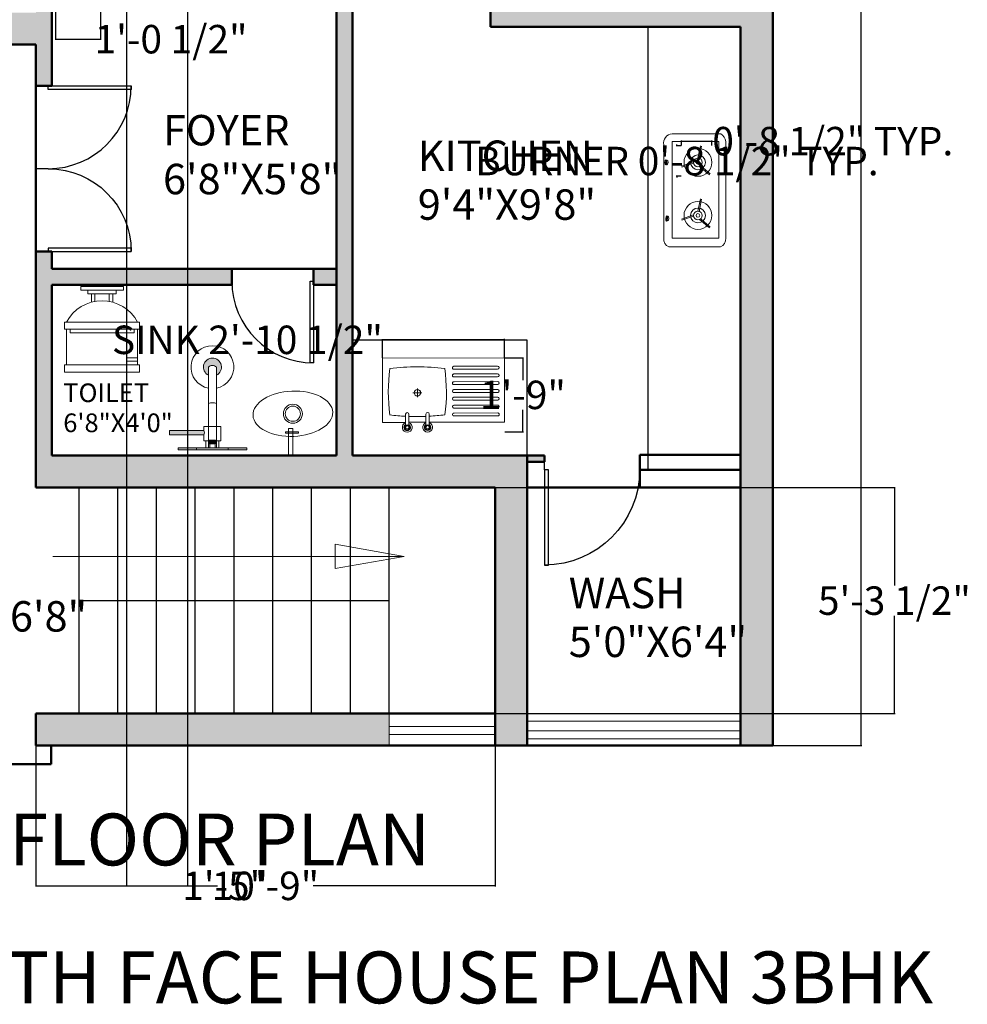
# Model space of a CAD drawing. Units: inches. Extents: x 22042254 to 25404563, y 17568978 to 17626777.
# Tile 36 of 45: x 22179932 to 22180198, y 17626125 to 17626402. Entities that reach past the tile are written whole.
import ezdxf

# ---------------------------------------------------------------- set-up
doc = ezdxf.new("R2010")
doc.units = ezdxf.units.IN
doc.header["$MEASUREMENT"] = 0
for name, color, linetype, lineweight in [('A-ANNO-DIMS', 2, 'Continuous', 18), ('A-ANNO-SYMB', 7, 'Continuous', 18), ('A-AREA-IDEN', 7, 'Continuous', 18), ('A-EQPM', 8, 'Continuous', 18), ('A-FLOR-CASE', 8, 'Continuous', 25), ('A-FLOR-STRS', 252, 'Continuous', 25), ('A-GLAZ', 4, 'Continuous', 18), ('A-WALL-PATT', 244, 'Continuous', 13), ('doors', 4, 'Continuous', 25), ('furniture', 8, 'Continuous', 18), ('PLUMBING FIXTURES', 9, 'Continuous', 18), ('text', 7, 'Continuous', 25), ('walls', 252, 'Continuous', 50)]:
    doc.layers.add(name, color=color, linetype=linetype, lineweight=lineweight)
doc.styles.get("Standard").update_dxf_attribs({"font": 'arial.ttf'})
doc.dimstyles.get("Standard").update_dxf_attribs({"dimtxt": 8, "dimasz": 0.18, "dimexe": 0.18, "dimexo": 0.0625, "dimgap": 0.09, "dimtad": 0, "dimtih": 1, "dimtoh": 1, "dimzin": 0, "dimdsep": 46, "dimlunit": 3, "dimtxsty": 'Standard', "dimcen": 0.09, "dimadec": 0, "dimazin": 0, "dimtfac": 1, "dimtofl": 0, "dimtmove": 0, "dimatfit": 3, "dimfxl": 1, "dimtolj": 1, "dimtzin": 0, "dimarcsym": 0})

# ---------------------------------------------------------------- blocks, each defined once
blk = doc.blocks.new('*D2')
at = {"layer": 'A-ANNO-DIMS', "color": 0, "lineweight": -2, "transparency": 16777216}
for p, q in [((22180143.8, 17626737.78), (22180168.82, 17626737.78)), ((22180168.64, 17626737.6), (22180168.64, 17626471.94)), ((22180168.64, 17626197.96), (22180168.64, 17626463.62)), ((22180143.8, 17626197.78), (22180168.82, 17626197.78))]:
    blk.add_line(p, q, dxfattribs=at)
at = {"layer": 'A-ANNO-DIMS', "color": 0, "transparency": 16777216}
for points in [[(22180168.61, 17626737.6), (22180168.67, 17626737.6), (22180168.64, 17626737.78)], [(22180168.61, 17626197.96), (22180168.67, 17626197.96), (22180168.64, 17626197.78)]]:
    blk.add_solid(points, dxfattribs=at)
at = {"layer": 'Defpoints', "color": 0, "transparency": 16777216}
for p in [(22180143.73, 17626737.78), (22180168.64, 17626737.78), (22180143.73, 17626197.78)]:
    blk.add_point(p, dxfattribs=at)
at = {"layer": 'A-ANNO-DIMS', "color": 0, "transparency": 16777216, "insert": (22180168.64, 17626467.78), "char_height": 8, "attachment_point": 5}
blk.add_mtext("\\A1;45'", dxfattribs=at)
blk = doc.blocks.new('A$C799204C7')
for p, q in [((0, 34.2), (17.99, 34.2)), ((0, 0), (0, 34.2)), ((17.99, 13.08), (17.99, 34.2)), ((2.32, 20.01), (2.32, 32.27)), ((3.13, 20.01), (3.13, 32.27)), ((4.48, 20.01), (4.48, 32.27)), ((5.29, 20.01), (5.29, 32.27)), ((6.64, 20.01), (6.64, 32.27)), ((7.45, 20.01), (7.45, 32.27)), ((8.85, 20.01), (8.85, 32.27)), ((9.66, 20.01), (9.66, 32.27)), ((11.01, 20.01), (11.01, 32.27)), ((11.82, 20.01), (11.82, 32.27)), ((13.22, 20.01), (13.22, 32.27)), ((14.03, 20.01), (14.03, 32.27)), ((15.42, 20.01), (15.42, 32.27)), ((16.24, 20.01), (16.24, 32.27)), ((18.59, 13.08), (15.71, 13.08)), ((15.71, 12.17), (18.59, 12.17)), ((17.99, 7.36), (17.99, 12.17)), ((8.52, 9.77), (10.9, 9.77)), ((9.73, 11), (9.73, 8.54)), ((18.59, 7.36), (15.71, 7.36)), ((15.71, 6.45), (18.59, 6.45)), ((17.99, 0), (17.99, 6.45)), ((0, 0), (17.99, 0))]:
    blk.add_line(p, q)
for centre, radius in [((19.38, 12.62), 0.684), ((19.38, 12.62), 0.456), ((9.7, 9.77), 0.916), ((19.38, 6.91), 0.684), ((19.38, 6.91), 0.456)]:
    blk.add_circle(centre, radius)
for centre, radius, start, end in [((2.72, 32.27), 0.407, 0, 180), ((4.88, 32.27), 0.407, 0, 180), ((7.05, 32.27), 0.407, 0, 180), ((9.25, 32.27), 0.407, 0, 180), ((11.42, 32.27), 0.407, 0, 180), ((13.62, 32.27), 0.407, 0, 180), ((15.83, 32.27), 0.407, 0, 180), ((2.72, 20.01), 0.407, 180, 0), ((4.88, 20.01), 0.407, 180, 0), ((7.05, 20.01), 0.407, 180, 0), ((9.25, 20.01), 0.407, 180, 0), ((11.42, 20.01), 0.407, 180, 0), ((13.62, 20.01), 0.407, 180, 0), ((15.83, 20.01), 0.407, 180, 0), ((67.33, 9.77), 64.88, 173.1952, 186.8048), ((9.53, -30.19), 48.1, 82.3437, 97.8966), ((-48.51, 9.77), 64.88, 2.9208, 6.8048), ((19.38, 12.62), 1.37, 199.6514, 160.3603), ((15.71, 12.62), 0.456, 90, 270), ((-48.51, 9.77), 64.88, 357.8723, 2.115), ((19.38, 12.62), 0.911, 210.3431, 149.7554), ((19.38, 6.91), 1.37, 199.6514, 160.3603), ((15.71, 6.91), 0.456, 90, 270), ((-48.51, 9.77), 64.88, 353.1952, 357.0665), ((19.38, 6.91), 0.911, 210.3431, 149.7554), ((9.53, 49.73), 48.1, 262.1034, 277.6563)]:
    blk.add_arc(centre, radius, start, end)
blk = doc.blocks.new('sink')
at = {"layer": 'furniture'}
for p, q in [((8718164203.894819, -1433730582.369047), (8718164201.504578, -1433730582.369047)), ((8718164202.684322, -1433730581.131674), (8718164202.684322, -1433730583.598095)), ((8718164196.150837, -1433730592.638258), (8718164196.150837, -1433730604.938997)), ((8718164196.967728, -1433730592.638258), (8718164196.967728, -1433730604.938997)), ((8718164198.365185, -1433730592.638258), (8718164198.365185, -1433730604.938997)), ((8718164199.182076, -1433730592.638258), (8718164199.182076, -1433730604.938997)), ((8718164200.579533, -1433730592.638258), (8718164200.579533, -1433730604.938997)), ((8718164201.396423, -1433730592.638258), (8718164201.396423, -1433730604.938997)), ((8718164202.748692, -1433730592.638258), (8718164202.748692, -1433730604.938997)), ((8718164203.565582, -1433730592.638258), (8718164203.565582, -1433730604.938997)), ((8718164204.963041, -1433730592.638258), (8718164204.963041, -1433730604.938997)), ((8718164205.779934, -1433730592.638258), (8718164205.779934, -1433730604.938997)), ((8718164207.1322, -1433730592.638258), (8718164207.1322, -1433730604.938997)), ((8718164207.949093, -1433730592.638258), (8718164207.949093, -1433730604.938997)), ((8718164209.301359, -1433730592.638258), (8718164209.301359, -1433730604.938997)), ((8718164210.118252, -1433730592.638258), (8718164210.118252, -1433730604.938997))]:
    blk.add_line(p, q, dxfattribs=at)
for centre, radius in [((8718164192.998869, -1433730579.495552), 0.685789), ((8718164192.998869, -1433730579.495552), 0.457192), ((8718164202.715019, -1433730582.369047), 0.919003), ((8718164192.998869, -1433730585.228166), 0.68579), ((8718164192.998869, -1433730585.228166), 0.68579), ((8718164192.998869, -1433730585.228166), 0.457192)]:
    blk.add_circle(centre, radius, dxfattribs=at)
for centre, radius, start, end in [((8718164196.559284, -1433730592.638258), 0.41045, 354.3355999, 185.6644001), ((8718164198.77363, -1433730592.638258), 0.41045, 354.3355999, 185.6644001), ((8718164200.98798, -1433730592.638258), 0.41045, 354.3355999, 185.6644001), ((8718164203.157139, -1433730592.638258), 0.41045, 354.3355999, 185.6644001), ((8718164205.371487, -1433730592.638258), 0.41045, 354.3355999, 185.6644001), ((8718164207.540646, -1433730592.640262), 0.41045, 354.3355999, 185.6644001), ((8718164209.709805, -1433730592.640262), 0.41045, 354.3355999, 185.6644001), ((8718164196.559284, -1433730604.938997), 0.408445, 180, 0), ((8718164198.77363, -1433730604.938997), 0.408445, 180, 0), ((8718164200.98798, -1433730604.938997), 0.408445, 180, 0), ((8718164203.157139, -1433730604.938997), 0.408445, 180, 0), ((8718164205.371487, -1433730604.938997), 0.408445, 180, 0), ((8718164207.540646, -1433730604.938997), 0.408445, 180, 0), ((8718164209.709805, -1433730604.938997), 0.408445, 180, 0)]:
    blk.add_arc(centre, radius, start, end, dxfattribs=at)
at = {"layer": 'furniture', "xscale": 1.0032, "yscale": 1.0032, "zscale": 1.0032, "rotation": 180}
blk.add_blockref('A$C799204C7', (8718164212.441259, -1433730572.566334), dxfattribs=at)
blk = doc.blocks.new('washbasin')
at = {"layer": 'furniture'}
blk.add_blockref('sink', (-8718164214.119328, 1433730589.721069), dxfattribs=at)
blk = doc.blocks.new('O.H SHOWER-PL')
at = {"layer": 'PLUMBING FIXTURES'}
for points in [[(-1.84, 0), (-1.84, -0.25), (1.84, -0.25), (1.84, 0)], [(0.46, -8.72), (0.46, -9.67, -0.422337), (-0.46, -9.67), (-0.46, -8.72, 4.325472)]]:
    blk.add_hatch(color=256, dxfattribs=at).paths.add_polyline_path(points)
for p, q in [((-1.84, 0), (-1.84, -0.25)), ((1.84, 0), (-1.84, 0)), ((1.84, 0), (1.84, -0.25)), ((1.84, -0.25), (-1.84, -0.25)), ((-0.46, -0.25), (-0.46, -9.67)), ((0.46, -0.25), (0.46, -9.67))]:
    blk.add_line(p, q, dxfattribs=at)
for centre, radius, start, end in [((0, -4.48), 1.03, 243.53, 296.47), ((0, -9.67), 2.5, 100.61, 79.39), ((0, -9.67), 1.05, 116.0349, 63.9652), ((0, -9.22), 0.643, 224.2078, 315.7922)]:
    blk.add_arc(centre, radius, start, end, dxfattribs=at)
blk = doc.blocks.new('DIVERTER-PL')
at = {"layer": 'PLUMBING FIXTURES'}
for points in [[(4, 0), (-4, 0), (-4, -0.25), (4, -0.25)], [(0.38, -1.14), (0.38, -0.7), (-0.37, -0.7), (-0.37, -1.14)], [(1, -1.75, 0.30818), (1, -2.25), (5, -2.25), (5, -1.75)]]:
    blk.add_hatch(color=256, dxfattribs=at).paths.add_polyline_path(points)
for p, q in [((-4, 0), (-4, -0.25)), ((-4, 0), (4, 0)), ((4, 0), (4, -0.25)), ((-4, -0.25), (4, -0.25)), ((-4, -0.25), (4, -0.25)), ((-1, -1.05), (-0.37, -1.05)), ((-1, -1.05), (-1, -2.75)), ((-0.75, -0.25), (-0.75, -1.05)), ((-0.37, -0.7), (0.38, -0.7)), ((-0.37, -0.7), (-0.37, -1.14)), ((-0.37, -1.14), (0.38, -1.14)), ((-0.32, -0.7), (-0.32, -0.25)), ((0.32, -0.7), (0.32, -0.25)), ((0.38, -0.7), (0.38, -1.14)), ((0.38, -1.05), (1, -1.05)), ((0.75, -0.25), (0.75, -1.05)), ((1, -1.05), (1, -1.75)), ((1, -2.25), (1, -2.75)), ((-1, -2.75), (1, -2.75))]:
    blk.add_line(p, q, dxfattribs=at)
at = {"layer": 'PLUMBING FIXTURES', "ltscale": 12}
for p, q in [((1, -1.75), (5, -1.75)), ((1, -2.25), (5, -2.25)), ((5, -2.25), (5, -1.75))]:
    blk.add_line(p, q, dxfattribs=at)
at = {"layer": 'PLUMBING FIXTURES'}
blk.add_arc((1.37, -2), 0.444, 145.7435, 214.2565, dxfattribs=at)
blk = doc.blocks.new('A$C7F153053')
at = {"layer": 'PLUMBING FIXTURES', "xscale": -1, "rotation": 270}
for name in ['DIVERTER-PL', 'O.H SHOWER-PL']:
    blk.add_blockref(name, (12.17, 4), dxfattribs=at)
blk = doc.blocks.new('Toilet - Imperial')
for p, q in [((-10, 22), (-10, 12)), ((-10, 21), (-7, 21)), ((-7, 20), (-10, 20)), ((-7, 21), (-7, 20)), ((10, 12), (10, 22)), ((10.5, 12), (-10.5, 12)), ((-10.5, 10), (-10.5, 12)), ((9, 13), (-9, 13)), ((-9, 13), (-9, 12)), ((9, 12), (9, 13)), ((10.5, 12), (10.5, 10)), ((10.5, 10), (-10.5, 10)), ((-3, 4.4065), (-3, 2)), ((-2, 2), (-2, 4.1658)), ((2, 4.1658), (2, 2)), ((3, 2), (3, 4.4065)), ((4, 2), (-4, 2)), ((-4, 2), (-4, 1)), ((4, 1), (4, 2))]:
    blk.add_line(p, q)
for points in [[(10.5, 22), (10.5, 24), (-10.5, 24), (-10.5, 22)], [(6, 0), (6, 1), (-6, 1), (-6, 0)]]:
    blk.add_lwpolyline(points, close=True)
blk.add_arc((0, 15.3333), 11.3333, 208.0725, 331.9275)
blk = doc.blocks.new('*U24')
for p, q in [((0, 0), (0, -6)), ((40, 0), (40, -6))]:
    blk.add_line(p, q)
blk.add_lwpolyline([(0, 0), (0, 40), (1.75, 40), (1.75, 0)], close=True)
blk.add_arc((0, 0), 40, 0, 90)
blk = doc.blocks.new('BASIN-OVAL-WITH-TAP')
for p, q in [((-11.77, 0), (-4.13, 0)), ((-5.47, 1.62), (-5.47, -2.04)), ((-5.06, 1.61), (-5.47, 1.61)), ((-5.06, -2.04), (-5.06, 1.61)), ((-4.13, 0), (-4.13, -1.24)), ((-4.13, -1.24), (-11.77, -1.24)), ((-5.47, -2.04), (-5.06, -2.04))]:
    blk.add_line(p, q)
for radius in [2.67, 2.13, 2.13, 2.13]:
    blk.add_circle((0, 0), radius)
blk.add_ellipse((0, 0), major_axis=(-0.46, -11.19), ratio=0.56899)
blk = doc.blocks.new('HOB-BURNER')
for p, q in [((0, 1.23), (0.68, 4.68)), ((0.33, 1.05), (0.97, 4.6)), ((-1.21, 0.17), (-4.61, -1.05)), ((-1.21, -0.2), (-4.53, -1.34)), ((0.46, -1.13), (3.22, -3.47)), ((0.78, -0.94), (3.43, -3.25))]:
    blk.add_line(p, q)
for radius in [3.91, 2.08, 1.22, 0.507]:
    blk.add_circle((0, 0), radius)
blk = doc.blocks.new('*D41')
at = {"layer": 'A-ANNO-DIMS', "color": 0, "lineweight": -2, "transparency": 16777216}
for p, q in [((22179942.23, 17626405.18), (22179942.23, 17626396.12)), ((22179954.87, 17626405.18), (22179954.87, 17626396.12)), ((22179942.41, 17626396.3), (22179954.69, 17626396.3)), ((22179954.87, 17626396.3), (22179955.05, 17626396.3))]:
    blk.add_line(p, q, dxfattribs=at)
at = {"layer": 'A-ANNO-DIMS', "color": 0, "transparency": 16777216}
for points in [[(22179942.41, 17626396.33), (22179942.41, 17626396.27), (22179942.23, 17626396.3)], [(22179954.69, 17626396.33), (22179954.69, 17626396.27), (22179954.87, 17626396.3)]]:
    blk.add_solid(points, dxfattribs=at)
at = {"layer": 'Defpoints', "color": 0, "transparency": 16777216}
for p in [(22179942.23, 17626405.24), (22179954.87, 17626405.24), (22179954.87, 17626396.3)]:
    blk.add_point(p, dxfattribs=at)
at = {"layer": 'A-ANNO-DIMS', "color": 0, "transparency": 16777216, "insert": (22179974.71, 17626396.3), "char_height": 8, "attachment_point": 5}
blk.add_mtext('\\A1;1\'-0 1/2"', dxfattribs=at)
blk = doc.blocks.new('*D54')
at = {"layer": 'A-ANNO-DIMS', "color": 0, "lineweight": -2, "transparency": 16777216}
for p, q in [((22180116.84, 17626366.54), (22180116.84, 17626366.72)), ((22180118.06, 17626366.36), (22180116.66, 17626366.36)), ((22180118.06, 17626357.77), (22180116.66, 17626357.77)), ((22180116.84, 17626357.59), (22180116.84, 17626357.41))]:
    blk.add_line(p, q, dxfattribs=at)
at = {"layer": 'A-ANNO-DIMS', "color": 0, "transparency": 16777216}
for points in [[(22180116.81, 17626366.54), (22180116.87, 17626366.54), (22180116.84, 17626366.36)], [(22180116.81, 17626357.59), (22180116.87, 17626357.59), (22180116.84, 17626357.77)]]:
    blk.add_solid(points, dxfattribs=at)
at = {"layer": 'Defpoints', "color": 0, "transparency": 16777216}
for p in [(22180116.84, 17626366.36), (22180118.13, 17626366.36), (22180118.13, 17626357.77)]:
    blk.add_point(p, dxfattribs=at)
at = {"layer": 'A-ANNO-DIMS', "color": 0, "transparency": 16777216, "insert": (22180116.84, 17626362.06), "char_height": 8, "attachment_point": 5}
blk.add_mtext('\\A1;BURNER 0\'-8 1/2" TYP.', dxfattribs=at)
blk = doc.blocks.new('*D55')
at = {"layer": 'A-ANNO-DIMS', "color": 0, "lineweight": -2, "transparency": 16777216}
for p, q in [((22180118.13, 17626366.42), (22180118.13, 17626367.83)), ((22180118.31, 17626367.65), (22180126.47, 17626367.65)), ((22180126.65, 17626366.42), (22180126.65, 17626367.83)), ((22180126.65, 17626367.65), (22180126.83, 17626367.65))]:
    blk.add_line(p, q, dxfattribs=at)
at = {"layer": 'A-ANNO-DIMS', "color": 0, "transparency": 16777216}
for points in [[(22180118.31, 17626367.68), (22180118.31, 17626367.62), (22180118.13, 17626367.65)], [(22180126.47, 17626367.68), (22180126.47, 17626367.62), (22180126.65, 17626367.65)]]:
    blk.add_solid(points, dxfattribs=at)
at = {"layer": 'Defpoints', "color": 0, "transparency": 16777216}
for p in [(22180126.65, 17626367.65), (22180118.13, 17626366.36), (22180126.65, 17626366.36)]:
    blk.add_point(p, dxfattribs=at)
at = {"layer": 'A-ANNO-DIMS', "color": 0, "transparency": 16777216, "insert": (22180160.62, 17626367.65), "char_height": 8, "attachment_point": 5}
blk.add_mtext('\\A1;0\'-8 1/2" TYP.', dxfattribs=at)
blk = doc.blocks.new('*D56')
at = {"layer": 'A-ANNO-DIMS', "color": 0, "lineweight": -2, "transparency": 16777216}
for p, q in [((22180034.08, 17626311.82), (22180033.9, 17626311.82)), ((22180034.09, 17626306.73), (22180034.08, 17626312)), ((22180068.21, 17626311.89), (22180034.26, 17626311.82)), ((22180068.4, 17626306.8), (22180068.39, 17626312.07))]:
    blk.add_line(p, q, dxfattribs=at)
at = {"layer": 'A-ANNO-DIMS', "color": 0, "transparency": 16777216}
for points in [[(22180034.26, 17626311.85), (22180034.26, 17626311.79), (22180034.08, 17626311.82)], [(22180068.21, 17626311.92), (22180068.21, 17626311.86), (22180068.39, 17626311.89)]]:
    blk.add_solid(points, dxfattribs=at)
at = {"layer": 'Defpoints', "color": 0, "transparency": 16777216}
for p in [(22180034.08, 17626311.82), (22180034.09, 17626306.67), (22180068.4, 17626306.74)]:
    blk.add_point(p, dxfattribs=at)
at = {"layer": 'A-ANNO-DIMS', "color": 0, "transparency": 16777216, "insert": (22179996.17, 17626311.82), "char_height": 8, "attachment_point": 5}
blk.add_mtext('\\A1;SINK 2\'-10 1/2"', dxfattribs=at)
blk = doc.blocks.new('*D57')
at = {"layer": 'A-ANNO-DIMS', "color": 0, "lineweight": -2, "transparency": 16777216}
for p, q in [((22180068.46, 17626306.74), (22180073.73, 17626306.75)), ((22180073.55, 17626306.57), (22180073.56, 17626300.52)), ((22180073.59, 17626286.12), (22180073.58, 17626292.17)), ((22180068.51, 17626285.93), (22180073.77, 17626285.94))]:
    blk.add_line(p, q, dxfattribs=at)
at = {"layer": 'A-ANNO-DIMS', "color": 0, "transparency": 16777216}
for points in [[(22180073.58, 17626306.57), (22180073.52, 17626306.57), (22180073.55, 17626306.75)], [(22180073.62, 17626286.12), (22180073.56, 17626286.12), (22180073.59, 17626285.94)]]:
    blk.add_solid(points, dxfattribs=at)
at = {"layer": 'Defpoints', "color": 0, "transparency": 16777216}
for p in [(22180068.4, 17626306.74), (22180073.55, 17626306.75), (22180068.44, 17626285.93)]:
    blk.add_point(p, dxfattribs=at)
at = {"layer": 'A-ANNO-DIMS', "color": 0, "transparency": 16777216, "insert": (22180073.57, 17626296.35), "char_height": 8, "attachment_point": 5}
blk.add_mtext('\\A1;1\'-9"', dxfattribs=at)
blk = doc.blocks.new('*D63')
at = {"layer": 'A-ANNO-DIMS', "color": 0, "lineweight": -2, "transparency": 16777216}
for p, q in [((22179962.22, 17626655.72), (22179962.22, 17626158.2)), ((22179979.38, 17626655.72), (22179979.38, 17626158.2)), ((22179962.4, 17626158.38), (22179979.2, 17626158.38)), ((22179979.38, 17626158.38), (22179979.56, 17626158.38))]:
    blk.add_line(p, q, dxfattribs=at)
at = {"layer": 'A-ANNO-DIMS', "color": 0, "transparency": 16777216}
for points in [[(22179962.4, 17626158.41), (22179962.4, 17626158.35), (22179962.22, 17626158.38)], [(22179979.2, 17626158.41), (22179979.2, 17626158.35), (22179979.38, 17626158.38)]]:
    blk.add_solid(points, dxfattribs=at)
at = {"layer": 'Defpoints', "color": 0, "transparency": 16777216}
for p in [(22179962.22, 17626655.78), (22179979.38, 17626655.78), (22179979.38, 17626158.38)]:
    blk.add_point(p, dxfattribs=at)
at = {"layer": 'A-ANNO-DIMS', "color": 0, "transparency": 16777216, "insert": (22179989.91, 17626158.38), "char_height": 8, "attachment_point": 5}
blk.add_mtext('\\A1;1\'-5"', dxfattribs=at)
blk = doc.blocks.new('*D64')
at = {"layer": 'A-ANNO-DIMS', "color": 0, "lineweight": -2, "transparency": 16777216}
for p, q in [((22180036.07, 17626270.28), (22180178.11, 17626270.28)), ((22180177.93, 17626270.1), (22180177.93, 17626242.76)), ((22180177.93, 17626206.96), (22180177.93, 17626234.3)), ((22180036.07, 17626206.78), (22180178.11, 17626206.78))]:
    blk.add_line(p, q, dxfattribs=at)
at = {"layer": 'A-ANNO-DIMS', "color": 0, "transparency": 16777216}
for points in [[(22180177.9, 17626270.1), (22180177.96, 17626270.1), (22180177.93, 17626270.28)], [(22180177.9, 17626206.96), (22180177.96, 17626206.96), (22180177.93, 17626206.78)]]:
    blk.add_solid(points, dxfattribs=at)
at = {"layer": 'Defpoints', "color": 0, "transparency": 16777216}
for p in [(22180036.01, 17626270.28), (22180036.01, 17626206.78), (22180177.93, 17626206.78)]:
    blk.add_point(p, dxfattribs=at)
at = {"layer": 'A-ANNO-DIMS', "color": 0, "transparency": 16777216, "insert": (22180177.93, 17626238.53), "char_height": 8, "attachment_point": 5}
blk.add_mtext('\\A1;5\'-3 1/2"', dxfattribs=at)
blk = doc.blocks.new('*D65')
at = {"layer": 'A-ANNO-DIMS', "color": 0, "lineweight": -2, "transparency": 16777216}
for p, q in [((22179936.73, 17626206.72), (22179936.73, 17626158.2)), ((22180065.73, 17626206.72), (22180065.73, 17626158.2)), ((22179936.91, 17626158.38), (22179987.78, 17626158.38)), ((22180065.55, 17626158.38), (22180014.69, 17626158.38))]:
    blk.add_line(p, q, dxfattribs=at)
at = {"layer": 'A-ANNO-DIMS', "color": 0, "transparency": 16777216}
for points in [[(22179936.91, 17626158.41), (22179936.91, 17626158.35), (22179936.73, 17626158.38)], [(22180065.55, 17626158.41), (22180065.55, 17626158.35), (22180065.73, 17626158.38)]]:
    blk.add_solid(points, dxfattribs=at)
at = {"layer": 'Defpoints', "color": 0, "transparency": 16777216}
for p in [(22179936.73, 17626206.78), (22180065.73, 17626206.78), (22180065.73, 17626158.38)]:
    blk.add_point(p, dxfattribs=at)
at = {"layer": 'A-ANNO-DIMS', "color": 0, "transparency": 16777216, "insert": (22180001.23, 17626158.38), "char_height": 8, "attachment_point": 5}
blk.add_mtext('\\A1;10\'-9"', dxfattribs=at)

msp = doc.modelspace()

# ---------------------------------------------------------------- hatches: boundary and pattern name
at = {"layer": 'A-WALL-PATT'}
h = msp.add_hatch(color=256, dxfattribs=at)
h.dxf.hatch_style = 1
h.paths.add_polyline_path([(22179792.734, 17626580.28), (22179888.734, 17626580.28), (22179888.734, 17626559.623), (22179893.234, 17626559.623), (22179893.234, 17626580.28), (22179900.438, 17626580.28), (22179900.438, 17626584.78), (22179792.734, 17626584.78), (22179792.734, 17626728.78), (22180134.734, 17626728.78), (22180134.734, 17626584.78), (22180035.602, 17626584.78), (22180004.432, 17626584.78), (22180001.734, 17626584.78), (22180001.734, 17626580.28), (22180134.734, 17626580.28), (22180134.734, 17626404.28), (22180064.487, 17626404.28), (22180064.487, 17626399.78), (22180134.734, 17626399.78), (22180134.734, 17626197.78), (22180143.734, 17626197.78), (22180143.734, 17626737.78), (22179783.734, 17626737.78), (22179783.734, 17626197.78), (22179792.734, 17626197.78), (22179792.734, 17626394.78), (22179936.734, 17626394.78), (22179936.734, 17626383.208), (22179941.234, 17626383.208), (22179941.234, 17626532.28), (22179927.066, 17626532.28), (22179927.066, 17626527.78), (22179928.072, 17626527.78), (22179936.734, 17626527.78), (22179936.734, 17626403.78), (22179792.734, 17626403.78), (22179792.734, 17626527.78), (22179905.094, 17626527.78), (22179905.094, 17626532.28), (22179792.734, 17626532.28)])
h = msp.add_hatch(color=256, dxfattribs=at)
h.dxf.hatch_style = 1
h.paths.add_polyline_path([(22179941.234, 17626336.599), (22179936.734, 17626336.599), (22179936.734, 17626270.28), (22180065.734, 17626270.28), (22180065.734, 17626197.78), (22180074.734, 17626197.78), (22180074.734, 17626279.28), (22180025.734, 17626279.28), (22180025.734, 17626404.28), (22180021.234, 17626404.28), (22180021.234, 17626279.28), (22179941.234, 17626279.28), (22179941.234, 17626327.28), (22179991.805, 17626327.28), (22179991.805, 17626331.78), (22179941.234, 17626331.78)])
h.paths.add_polyline_path([(22180036.005, 17626206.78), (22179936.734, 17626206.78), (22179936.734, 17626197.78), (22180036.005, 17626197.78)], flags=17)
h.paths.add_polyline_path([(22179836.995, 17626451.976), (22179902.189, 17626451.976), (22179902.189, 17626465.064), (22179836.995, 17626465.064)], flags=9)
h.paths.add_polyline_path([(22179836.966, 17626465.674), (22179903.069, 17626465.674), (22179903.069, 17626478.937), (22179836.966, 17626478.937)], flags=9)
h.paths.add_polyline_path([(22180055.036, 17626649.533), (22180120.23, 17626649.533), (22180120.23, 17626662.622), (22180055.036, 17626662.622)], flags=9)
h.paths.add_polyline_path([(22180055.007, 17626663.231), (22180121.111, 17626663.231), (22180121.111, 17626676.495), (22180055.007, 17626676.495)], flags=9)
h = msp.add_hatch(color=256, dxfattribs=at)
h.dxf.hatch_style = 1
h.paths.add_polyline_path([(22179893.234, 17626536.599), (22179889.78, 17626536.599), (22179888.734, 17626536.599), (22179888.734, 17626532.28), (22179893.234, 17626532.28)], flags=17)
h.paths.add_polyline_path([(22180021.234, 17626331.78), (22180014.784, 17626331.78), (22180014.784, 17626328.329), (22180014.784, 17626327.28), (22180021.234, 17626327.28)], flags=17)
h.paths.add_polyline_path([(22180079.631, 17626279.28), (22180074.734, 17626279.28), (22180074.734, 17626277.567), (22180079.631, 17626277.567)], flags=17)
h.paths.add_polyline_path([(22179935.729, 17626503.598), (22179935.729, 17626431.832), (22179920.515, 17626431.832), (22179920.515, 17626503.598)], flags=0)
h.paths.add_polyline_path([(22179931.81, 17626498.421), (22179931.81, 17626479.569), (22179933.631, 17626479.569, -0.4142136), (22179934.711, 17626478.489), (22179934.711, 17626457.445, -0.4142136), (22179933.631, 17626456.365), (22179931.81, 17626456.365), (22179931.81, 17626437.513), (22179930.36, 17626437.513, -0.0640419), (22179928.185, 17626440.982), (22179928.185, 17626456.365), (22179927.814, 17626456.365, -0.4142136), (22179926.735, 17626457.445), (22179926.735, 17626478.489, -0.4142136), (22179927.814, 17626479.569), (22179928.185, 17626479.569), (22179928.185, 17626494.952, -0.0640419), (22179930.36, 17626498.421)], flags=0)
h.paths.add_polyline_path([(22179869.738, 17626505.187), (22179869.738, 17626429.601), (22179838.221, 17626429.601), (22179838.221, 17626437.096), (22179809.382, 17626437.096), (22179809.505, 17626424.396), (22179794.94, 17626424.396), (22179794.818, 17626437.096), (22179794.818, 17626493.783), (22179794.695, 17626506.484), (22179809.26, 17626506.484), (22179809.382, 17626493.783), (22179838.221, 17626493.783), (22179838.221, 17626505.187)], flags=0)
h.paths.add_polyline_path([(22179814.199, 17626493.722), (22179814.199, 17626483.494), (22179806.658, 17626483.494), (22179806.607, 17626483.426), (22179806.607, 17626443.497), (22179798.041, 17626443.497), (22179798.041, 17626460.107), (22179806.607, 17626460.107), (22179806.607, 17626466.884), (22179798.041, 17626466.884), (22179798.041, 17626483.494), (22179806.658, 17626483.494)], flags=0)
h.paths.add_polyline_path([(22179806.666, 17626500.475, -1), (22179797.289, 17626500.475, -1)], flags=0)
h.paths.add_polyline_path([(22179806.789, 17626431.088, -1), (22179797.412, 17626431.088, -1)], flags=0)
h.paths.add_polyline_path([(22179836.995, 17626451.976), (22179902.189, 17626451.976), (22179902.189, 17626465.064), (22179836.995, 17626465.064)], flags=8)
h.paths.add_polyline_path([(22179836.966, 17626465.674), (22179903.069, 17626465.674), (22179903.069, 17626478.937), (22179836.966, 17626478.937)], flags=8)

# ---------------------------------------------------------------- linework, layer by layer
at = {"layer": 'A-ANNO-SYMB'}
for p, q in [((22180020.858, 17626250.979), (22180020.858, 17626254.397)), ((22180020.858, 17626254.397), (22180040.181, 17626250.979)), ((22179941.541, 17626250.979), (22180020.858, 17626250.979)), ((22180020.858, 17626250.979), (22180040.181, 17626250.979)), ((22180020.858, 17626250.979), (22180020.858, 17626247.561)), ((22180020.858, 17626247.561), (22180040.181, 17626250.979))]:
    msp.add_line(p, q, dxfattribs=at)
at = {"layer": 'A-EQPM'}
for p, q in [((22180129.13, 17626369.703), (22180115.508, 17626369.703)), ((22180113.114, 17626366.626), (22180113.114, 17626340.389)), ((22180128.649, 17626367.562), (22180115.508, 17626367.562)), ((22180115.508, 17626367.562), (22180115.508, 17626340.389)), ((22180128.649, 17626340.389), (22180128.649, 17626367.562)), ((22180130.533, 17626367.562), (22180130.533, 17626340.389)), ((22180115.508, 17626340.389), (22180128.649, 17626340.389)), ((22180129.056, 17626337.942), (22180114.521, 17626337.942))]:
    msp.add_line(p, q, dxfattribs=at)
for centre, radius, start, end in [((22180115.687, 17626367.094), 2.615, 93.92707, 190.30452), ((22180127.924, 17626367.382), 2.615, 3.92707, 62.5308), ((22180115.505, 17626340.135), 2.404, 173.93636, 246.89401), ((22180128.14, 17626340.165), 2.404, 292.40616, 5.36382)]:
    msp.add_arc(centre, radius, start, end, dxfattribs=at)
for centre, major_axis, ratio in [((22180113.735, 17626361.686), (0.02, 0.713), 0.3769734), ((22180114.004, 17626361.679), (0.043, 0.664), 0.4928397), ((22180113.963, 17626345.916), (0.02, 0.713), 0.3769734), ((22180114.232, 17626345.909), (0.043, 0.664), 0.4928397)]:
    msp.add_ellipse(centre, major_axis=major_axis, ratio=ratio, dxfattribs=at)
at = {"layer": 'A-FLOR-CASE'}
for p, q in [((22180108.757, 17626275.269), (22180108.757, 17626399.78)), ((22180074.734, 17626311.701), (22180025.734, 17626311.701)), ((22180074.734, 17626279.28), (22180074.734, 17626311.701))]:
    msp.add_line(p, q, dxfattribs=at)
at = {"layer": 'A-FLOR-STRS'}
for p, q in [((22179948.859, 17626206.78), (22179948.859, 17626270.28)), ((22179959.752, 17626206.78), (22179959.752, 17626270.28)), ((22179970.646, 17626206.78), (22179970.646, 17626270.28)), ((22179981.539, 17626206.78), (22179981.539, 17626270.28)), ((22179992.432, 17626206.78), (22179992.432, 17626270.28)), ((22180003.326, 17626206.78), (22180003.326, 17626270.28)), ((22180014.219, 17626206.78), (22180014.219, 17626270.28)), ((22180025.112, 17626206.78), (22180025.112, 17626270.28)), ((22180036.005, 17626206.78), (22180036.005, 17626270.28)), ((22179948.859, 17626238.53), (22180036.005, 17626238.53))]:
    msp.add_line(p, q, dxfattribs=at)
at = {"layer": 'A-GLAZ'}
for p, q in [((22180036.005, 17626206.78), (22180036.005, 17626197.78)), ((22180065.734, 17626206.78), (22180036.005, 17626206.78)), ((22180036.005, 17626206.78), (22180036.005, 17626203.194)), ((22180065.734, 17626197.78), (22180065.734, 17626206.78)), ((22180074.734, 17626204.648), (22180134.734, 17626204.648)), ((22180134.734, 17626204.648), (22180134.734, 17626201.966)), ((22180036.005, 17626203.194), (22180065.734, 17626203.194)), ((22180065.734, 17626200.938), (22180036.005, 17626200.938)), ((22180065.734, 17626203.194), (22180065.734, 17626200.938)), ((22180134.734, 17626201.966), (22180074.734, 17626201.966)), ((22180074.734, 17626201.966), (22180074.734, 17626199.741)), ((22180074.734, 17626199.741), (22180134.734, 17626199.741)), ((22180036.005, 17626197.78), (22180065.734, 17626197.78))]:
    msp.add_line(p, q, dxfattribs=at)
at = {"layer": 'walls'}
for p, q in [((22180143.734, 17626737.78), (22180143.734, 17626197.78)), ((22179941.234, 17626383.208), (22179941.234, 17626532.28)), ((22180021.234, 17626279.28), (22180021.234, 17626404.28)), ((22180025.734, 17626279.28), (22180025.734, 17626404.28)), ((22180064.487, 17626404.28), (22180064.487, 17626399.78)), ((22180064.487, 17626399.78), (22180134.734, 17626399.78)), ((22180134.734, 17626399.78), (22180134.734, 17626197.78)), ((22179792.734, 17626394.78), (22179936.734, 17626394.78)), ((22179936.734, 17626270.28), (22179936.734, 17626394.78)), ((22179936.734, 17626383.208), (22179941.234, 17626383.208)), ((22179936.734, 17626336.599), (22179941.234, 17626336.599)), ((22179941.234, 17626331.78), (22179941.234, 17626336.599)), ((22179941.234, 17626331.78), (22180021.234, 17626331.78)), ((22179991.805, 17626327.28), (22179991.805, 17626331.78)), ((22180014.784, 17626327.28), (22180014.784, 17626331.78)), ((22179941.234, 17626279.28), (22179941.234, 17626327.28)), ((22179941.234, 17626327.28), (22179991.805, 17626327.28)), ((22179941.234, 17626279.28), (22179941.234, 17626327.28)), ((22180014.784, 17626327.28), (22180021.234, 17626327.28)), ((22179941.234, 17626279.28), (22180021.234, 17626279.28)), ((22180025.734, 17626279.28), (22180074.734, 17626279.28)), ((22180074.734, 17626279.28), (22180074.734, 17626197.78)), ((22180074.734, 17626279.28), (22180079.631, 17626279.28)), ((22180079.631, 17626277.567), (22180079.631, 17626279.28)), ((22180106.37, 17626279.529), (22180106.37, 17626275.269)), ((22180134.734, 17626279.529), (22180106.37, 17626279.529)), ((22180134.734, 17626275.269), (22180134.734, 17626279.529)), ((22180074.734, 17626277.567), (22180079.631, 17626277.567)), ((22180106.37, 17626275.269), (22180106.37, 17626270.28)), ((22180106.37, 17626275.269), (22180134.734, 17626275.269)), ((22179936.734, 17626270.28), (22180065.734, 17626270.28)), ((22180065.734, 17626270.28), (22180065.734, 17626197.78)), ((22180074.734, 17626270.28), (22180134.734, 17626270.28)), ((22179936.734, 17626197.78), (22179936.734, 17626206.78)), ((22180065.734, 17626206.78), (22179936.734, 17626206.78)), ((22180143.734, 17626197.78), (22179936.734, 17626197.78)), ((22179941.027, 17626192.584), (22179941.027, 17626197.78)), ((22179783.734, 17626192.584), (22179936.734, 17626192.584)), ((22179936.734, 17626192.584), (22179941.027, 17626192.584))]:
    msp.add_line(p, q, dxfattribs=at)

# ---------------------------------------------------------------- block references
at = {"layer": 'A-EQPM'}
for p in [(22180122.74, 17626361.682), (22180122.74, 17626346.769)]:
    msp.add_blockref('HOB-BURNER', p, dxfattribs=at)
at = {"layer": 'doors'}
for p, xscale, yscale, zscale, rotation in [((22179940.229, 17626383.208), 0.5826086806699359, 0.5826086806699359, 0.5826086806699359, 270), ((22179940.229, 17626336.599), -0.5826086806699359, 0.5826086806699359, 0.5826086806699359, 270), ((22180014.784, 17626328.329), 0.5750671146789703, 0.5750671146789703, 0.5750671146789703, 180), ((22180079.631, 17626275.269), -0.6684818809186152, 0.6684818809186152, 0.6684818809186152, 180)]:
    msp.add_blockref('*U24', p, dxfattribs=dict(at, xscale=xscale, yscale=yscale, zscale=zscale, rotation=rotation))
at = {"layer": 'PLUMBING FIXTURES'}
for name, p, rotation in [('Toilet - Imperial', (22179955.33, 17626326.78), 180), ('washbasin', (22180051.243, 17626308.384), 90.12017160754561)]:
    msp.add_blockref(name, p, dxfattribs=dict(at, rotation=rotation))
at = {"layer": 'PLUMBING FIXTURES', "xscale": -2.406230429091579, "yscale": 2.406230429091579, "zscale": 2.406230429091579, "rotation": 90}
msp.add_blockref('A$C7F153053', (22179995.964, 17626310.175), dxfattribs=at)
at = {"layer": 'PLUMBING FIXTURES', "extrusion": (0, 0, -1), "zscale": -1, "rotation": 89.99999988950991}
msp.add_blockref('BASIN-OVAL-WITH-TAP', (-22180008.933, 17626291.052), dxfattribs=at)

# ---------------------------------------------------------------- texts
at = {"layer": 'A-AREA-IDEN'}
for s, height, p in [('FOYER', 8.5453, (22179972.46, 17626366.459)), ('KITCHEN', 8.5453, (22180044.031, 17626359.284)), ('6\'8"X5\'8"', 8.5453, (22179972.46, 17626352.732)), ('9\'4"X9\'8"', 8.5453, (22180044.031, 17626345.557)), ('TOILET', 5.248, (22179944.444, 17626294.308)), ('6\'8"X4\'0"', 5.248, (22179944.444, 17626285.878)), ('WASH', 8.5453, (22180086.456, 17626236.415)), ('12\'0"X16\'8"', 8.54529, (22179888.134, 17626229.838)), ('5\'0"X6\'4"', 8.5453, (22180086.456, 17626222.687))]:
    msp.add_text(s, height=height, dxfattribs=at).set_placement(p)
at = {"layer": 'text'}
for s, p in [('GROUND FLOOR PLAN', (22179841.196, 17626164.124)), ('30X45 SOUTH FACE HOUSE PLAN 3BHK', (22179827.516, 17626125.358))]:
    msp.add_text(s, height=14.58777, dxfattribs=at).set_placement(p)

# ---------------------------------------------------------------- dimensions: what is measured, and where the dimension line sits
at = {"layer": 'A-ANNO-DIMS'}
for base, p1, p2, angle, override, picture, middle in [((22180168.64, 17626737.78), (22180143.734, 17626197.78), (22180143.734, 17626737.78), 90, {"dimclrd": 0, "dimclre": 0, "dimclrt": 0}, '*D2', (22180168.64, 17626467.78)), ((22180073.547, 17626306.753), (22180068.445, 17626285.928), (22180068.401, 17626306.742), 90.12017, {"dimdec": 1, "dimlfac": 1, "dimrnd": 0, "dimzin": 1, "dimdsep": 46, "dimlunit": 4, "dimfrac": 2}, '*D57', (22180073.569, 17626296.346)), ((22180177.934, 17626206.78), (22180036.005, 17626270.28), (22180036.005, 17626206.78), 90, {"dimdec": 1, "dimlfac": 1, "dimrnd": 0, "dimzin": 1, "dimdsep": 46, "dimlunit": 4, "dimfrac": 2}, '*D64', (22180177.934, 17626238.53))]:
    dim = msp.add_linear_dim(base=base, p1=p1, p2=p2, angle=angle, dimstyle='Standard', override=override, dxfattribs=at)
    dim.commit()
    dim.dimension.update_dxf_attribs({"geometry": picture, "text_midpoint": middle})
for base, p1, p2, picture, middle in [((22179979.384, 17626158.384), (22179962.224, 17626655.782), (22179979.384, 17626655.782), '*D63', (22179989.911, 17626158.384)), ((22179954.866, 17626396.301), (22179942.234, 17626405.239), (22179954.866, 17626405.239), '*D41', (22179974.713, 17626396.301)), ((22180065.734, 17626158.384), (22179936.734, 17626206.78), (22180065.734, 17626206.78), '*D65', (22180001.234, 17626158.384))]:
    dim = msp.add_linear_dim(base=base, p1=p1, p2=p2, dimstyle='Standard', override={"dimdec": 1, "dimlfac": 1, "dimrnd": 0, "dimzin": 1, "dimdsep": 46, "dimlunit": 4, "dimfrac": 2}, dxfattribs=at)
    dim.commit()
    dim.dimension.update_dxf_attribs({"geometry": picture, "text_midpoint": middle})
for base, p1, p2, angle, text, picture, middle in [((22180116.838, 17626366.358), (22180118.126, 17626357.77), (22180118.126, 17626366.358), 90, 'BURNER <> TYP.', '*D54', (22180116.838, 17626362.064)), ((22180034.081, 17626311.816), (22180068.401, 17626306.742), (22180034.092, 17626306.67), 180.12017, 'SINK <>', '*D56', (22179996.174, 17626311.816))]:
    dim = msp.add_linear_dim(base=base, p1=p1, p2=p2, angle=angle, text=text, dimstyle='Standard', override={"dimdec": 1, "dimlfac": 1, "dimrnd": 0, "dimzin": 1, "dimdsep": 46, "dimlunit": 4, "dimfrac": 2}, dxfattribs=at)
    dim.commit()
    dim.dimension.update_dxf_attribs({"geometry": picture, "text_midpoint": middle})
dim = msp.add_linear_dim(base=(22180126.652, 17626367.646), p1=(22180118.126, 17626366.358), p2=(22180126.652, 17626366.358), text='<> TYP.', dimstyle='Standard', override={"dimdec": 1, "dimlfac": 1, "dimrnd": 0, "dimzin": 1, "dimdsep": 46, "dimlunit": 4, "dimfrac": 2}, dxfattribs=at)
dim.commit()
dim.dimension.update_dxf_attribs({"geometry": '*D55', "text_midpoint": (22180160.625, 17626367.646)})

doc.saveas('drawing.dxf')
